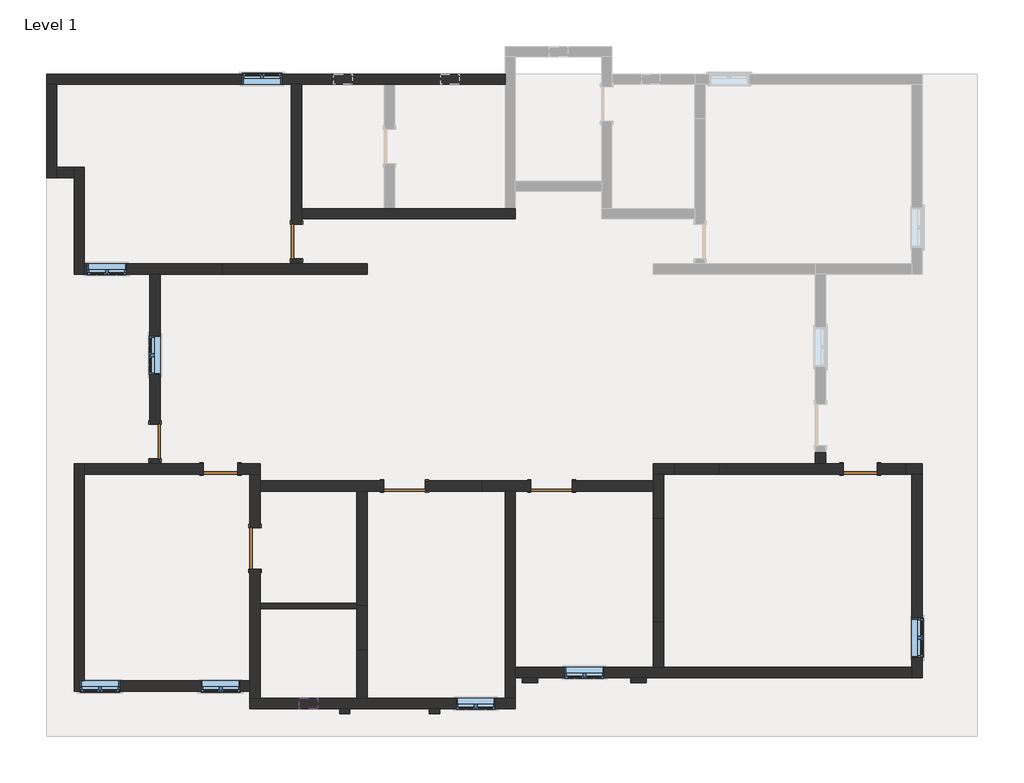
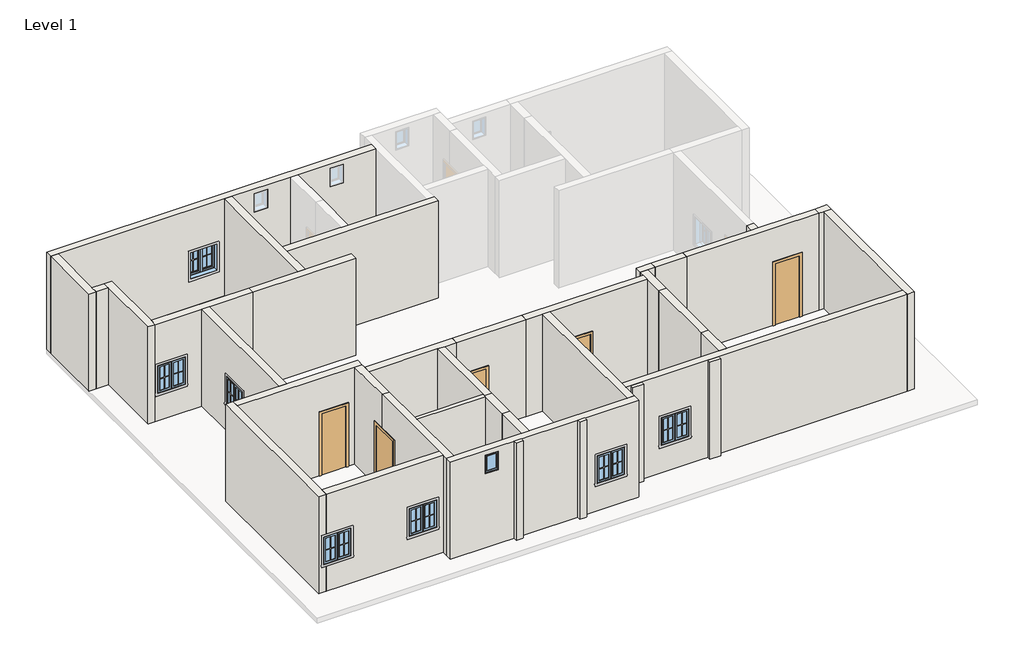
# One storey, part 1 of 2: 37 walls, 9 windows, 7 doors.
"""IFC4 building model written with IfcOpenShell, lengths in millimetres."""

from ifc_helpers import new_model, si_unit, frame, origin, origin_with_axes, place, context, project, spatial, polyline, outline, extrude, faceted_brep, transform, mapped, element, save
from components import door_a1484949, door_85036156, door_89fc3733, window_aa618e30, window_339605e1, window_791baf9d

model = new_model("IFC4")

# Units and contexts
model_context = context("Model", 3, world=origin())
ifc_project = project(units=[si_unit("LENGTHUNIT", "METRE", prefix="MILLI")], contexts=[model_context])

# Site, building, storey
site = spatial("IfcSite", under=ifc_project)
building = spatial("IfcBuilding", under=site)
storey = spatial("IfcBuildingStorey", under=building, Name="Level 1", Elevation=0.0)

# Doors
placement = place(None, origin())
door_shape = door_a1484949(model_context)
element("IfcDoor", 1, ObjectType="Single-Flush : 30\" x 80\"", at=placement, inside=storey, context=model_context, shape_type="MappedRepresentation", body=[
    mapped(door_shape, transform((-11694.6415084, -147.6064015, 0.0), x_axis=(0.0, -1.0, 0.0), y_axis=(1.0, 0.0, 0.0), z_axis=(0.0, 0.0, 1.0))),
])
door_2_shape = door_85036156(model_context)
element("IfcDoor", 2, ObjectType="Single-Flush : 30\" x 80\"", at=placement, inside=storey, context=model_context, shape_type="MappedRepresentation", body=[
    mapped(door_2_shape, transform((-8570.4415084, 4271.9935985, 0.0), x_axis=(0.0, -1.0, 0.0), y_axis=(1.0, 0.0, 0.0), z_axis=(0.0, 0.0, 1.0))),
])
element("IfcDoor", 3, ObjectType="Single-Flush : 30\" x 80\"", at=placement, inside=storey, context=model_context, shape_type="MappedRepresentation", body=[
    mapped(door_2_shape, transform((-10246.8415084, -757.2064015, 0.0), x_axis=(1.0, 0.0, 0.0), y_axis=(0.0, 1.0, 0.0), z_axis=(0.0, 0.0, 1.0))),
])
element("IfcDoor", 4, ObjectType="Single-Flush : 30\" x 80\"", at=placement, inside=storey, context=model_context, shape_type="MappedRepresentation", body=[
    mapped(door_2_shape, transform((3888.6257783, -757.2064015, 0.0), x_axis=(1.0, 0.0, 0.0), y_axis=(0.0, 1.0, 0.0), z_axis=(0.0, 0.0, 1.0))),
])
door_3_shape = door_89fc3733(model_context)
element("IfcDoor", 5, ObjectType="Single-Flush : 36\" x 80\"", at=placement, inside=storey, context=model_context, shape_type="MappedRepresentation", body=[
    mapped(door_3_shape, transform((-9484.8415084, -2515.5755761, 0.0), x_axis=(0.0, 1.0, 0.0), y_axis=(-1.0, 0.0, 0.0), z_axis=(0.0, 0.0, 1.0))),
])
element("IfcDoor", 6, ObjectType="Single-Flush : 36\" x 80\"", at=placement, inside=storey, context=model_context, shape_type="MappedRepresentation", body=[
    mapped(door_3_shape, transform((-6181.702216, -1138.2064015, 0.0), x_axis=(-1.0, 0.0, 0.0), y_axis=(0.0, -1.0, 0.0), z_axis=(0.0, 0.0, 1.0))),
])
element("IfcDoor", 7, ObjectType="Single-Flush : 36\" x 80\"", at=placement, inside=storey, context=model_context, shape_type="MappedRepresentation", body=[
    mapped(door_3_shape, transform((-2931.6415084, -1138.2064015, 0.0), x_axis=(-1.0, 0.0, 0.0), y_axis=(0.0, -1.0, 0.0), z_axis=(0.0, 0.0, 1.0))),
])

# Walls
element("IfcWall", 8, ObjectType="4.5\"", at=placement, inside=storey, context=model_context, shape_type="Brep", body=[
    faceted_brep([(-9370.5415084, -3843.3848078, 0.0), (-7236.9415084, -3843.3848078, 0.0), (-7236.9415084, -3843.3848078, 3200.4), (-9370.5415084, -3843.3848078, 3200.4), (-9370.5415084, -3729.0848078, 0.0), (-9370.5415084, -3729.0848078, 3200.4), (-7236.9415084, -3729.0848078, 3200.4), (-7236.9415084, -3729.0848078, 0.0), (-7236.9415084, -3786.2348078, 0.0), (-7236.9415084, -3786.2348078, 3200.4)], [[[0, 1, 2, 3]], [[4, 5, 6, 7]], [[1, 0, 4, 7, 8]], [[3, 2, 9, 6, 5]], [[2, 1, 8, 7, 6, 9]], [[0, 3, 5, 4]]]),
])
element("IfcWall", 9, ObjectType="4.5\"", at=placement, inside=storey, context=model_context, shape_type="SweptSolid", body=[
    extrude(outline(polyline([(-7389.3415084, -6167.4848078), (-7617.9415084, -6167.4848078), (-7617.9415084, -6053.1848078), (-7389.3415084, -6053.1848078), (-7389.3415084, -6167.4848078)])), origin_with_axes(), (0.0, 0.0, 1.0), 3200.4),
])
element("IfcWall", 10, ObjectType="4.5\"", at=placement, inside=storey, context=model_context, shape_type="SweptSolid", body=[
    extrude(outline(polyline([(-5408.1415084, -6167.4848078), (-5636.7415084, -6167.4848078), (-5636.7415084, -6053.1848078), (-5408.1415084, -6053.1848078), (-5408.1415084, -6167.4848078)])), origin_with_axes(), (0.0, 0.0, 1.0), 3200.4),
])
element("IfcWall", 11, ObjectType="4.5\"", at=placement, inside=storey, context=model_context, shape_type="SweptSolid", body=[
    extrude(outline(polyline([(-3236.4415084, -5481.6064015), (-3579.3415084, -5481.6064015), (-3579.3415084, -5367.3064015), (-3236.4415084, -5367.3064015), (-3236.4415084, -5481.6064015)])), origin_with_axes(), (0.0, 0.0, 1.0), 3200.4),
])
element("IfcWall", 12, ObjectType="4.5\"", at=placement, inside=storey, context=model_context, shape_type="SweptSolid", body=[
    extrude(outline(polyline([(-836.1415084, -5481.6064015), (-1179.0415084, -5481.6064015), (-1179.0415084, -5367.3064015), (-836.1415084, -5367.3064015), (-836.1415084, -5481.6064015)])), origin_with_axes(), (0.0, 0.0, 1.0), 3200.4),
])
element("IfcWall", 13, ObjectType="9\"", at=placement, inside=storey, context=model_context, shape_type="Brep", body=[
    faceted_brep([(-3960.3415084, 7967.6935985, 0.0), (-14094.9415084, 7967.6935985, 0.0), (-14094.9415084, 7967.6935985, 3200.4), (-3960.3415084, 7967.6935985, 3200.4), (-8900.6415084, 7967.6935985, 1828.8), (-9764.2415084, 7967.6935985, 1828.8), (-9764.2415084, 7967.6935985, 914.4), (-8900.6415084, 7967.6935985, 914.4), (-7338.5415084, 7967.6935985, 3048.0), (-7744.9415084, 7967.6935985, 3048.0), (-7744.9415084, 7967.6935985, 2438.4), (-7338.5415084, 7967.6935985, 2438.4), (-4976.3415084, 7967.6935985, 3048.0), (-5382.7415084, 7967.6935985, 3048.0), (-5382.7415084, 7967.6935985, 2438.4), (-4976.3415084, 7967.6935985, 2438.4), (-3960.3415084, 7739.0935985, 0.0), (-3960.3415084, 7739.0935985, 3200.4), (-6398.7415084, 7739.0935985, 3200.4), (-6627.3415084, 7739.0935985, 3200.4), (-8456.1415084, 7739.0935985, 3200.4), (-8684.7415084, 7739.0935985, 3200.4), (-13866.3415084, 7739.0935985, 3200.4), (-14094.9415084, 7739.0935985, 3200.4), (-14094.9415084, 7739.0935985, 0.0), (-13866.3415084, 7739.0935985, 0.0), (-8684.7415084, 7739.0935985, 0.0), (-8456.1415084, 7739.0935985, 0.0), (-6627.3415084, 7739.0935985, 0.0), (-6398.7415084, 7739.0935985, 0.0), (-8900.6415084, 7739.0935985, 1828.8), (-8900.6415084, 7739.0935985, 914.4), (-9764.2415084, 7739.0935985, 914.4), (-9764.2415084, 7739.0935985, 1828.8), (-7338.5415084, 7739.0935985, 3048.0), (-7338.5415084, 7739.0935985, 2438.4), (-7744.9415084, 7739.0935985, 2438.4), (-7744.9415084, 7739.0935985, 3048.0), (-4976.3415084, 7739.0935985, 3048.0), (-4976.3415084, 7739.0935985, 2438.4), (-5382.7415084, 7739.0935985, 2438.4), (-5382.7415084, 7739.0935985, 3048.0)], [[[0, 1, 2, 3], [4, 5, 6, 7], [8, 9, 10, 11], [12, 13, 14, 15]], [[16, 17, 18, 19, 20, 21, 22, 23, 24, 25, 26, 27, 28, 29], [30, 31, 32, 33], [34, 35, 36, 37], [38, 39, 40, 41]], [[1, 0, 16, 29, 28, 27, 26, 25, 24]], [[3, 2, 23, 22, 21, 20, 19, 18, 17]], [[2, 1, 24, 23]], [[0, 3, 17, 16]], [[31, 30, 4, 7]], [[32, 31, 7, 6]], [[33, 32, 6, 5]], [[30, 33, 5, 4]], [[35, 34, 8, 11]], [[36, 35, 11, 10]], [[37, 36, 10, 9]], [[34, 37, 9, 8]], [[39, 38, 12, 15]], [[40, 39, 15, 14]], [[41, 40, 14, 13]], [[38, 41, 13, 12]]]),
])
element("IfcWall", 14, ObjectType="9\"", at=placement, inside=storey, context=model_context, shape_type="Brep", body=[
    faceted_brep([(-14094.9415084, 7739.0935985, 0.0), (-14094.9415084, 5681.6935985, 0.0), (-14094.9415084, 5681.6935985, 3200.4), (-14094.9415084, 7739.0935985, 3200.4), (-13866.3415084, 7739.0935985, 0.0), (-13866.3415084, 7739.0935985, 3200.4), (-13866.3415084, 5910.2935985, 3200.4), (-13866.3415084, 5681.6935985, 3200.4), (-13866.3415084, 5681.6935985, 0.0), (-13866.3415084, 5910.2935985, 0.0)], [[[0, 1, 2, 3]], [[4, 5, 6, 7, 8, 9]], [[1, 0, 4, 9, 8]], [[3, 2, 7, 6, 5]], [[0, 3, 5, 4]], [[2, 1, 8, 7]]]),
])
element("IfcWall", 15, ObjectType="9\"", at=placement, inside=storey, context=model_context, shape_type="Brep", body=[
    faceted_brep([(-13485.3415084, 5910.2935985, 0.0), (-13485.3415084, 5681.6935985, 0.0), (-13485.3415084, 3548.0935985, 0.0), (-13485.3415084, 3548.0935985, 3200.4), (-13485.3415084, 5681.6935985, 3200.4), (-13485.3415084, 5910.2935985, 3200.4), (-13256.7415084, 5910.2935985, 0.0), (-13256.7415084, 5910.2935985, 3200.4), (-13256.7415084, 3776.6935985, 3200.4), (-13256.7415084, 3548.0935985, 3200.4), (-13256.7415084, 3548.0935985, 0.0), (-13256.7415084, 3776.6935985, 0.0)], [[[0, 1, 2, 3, 4, 5]], [[6, 7, 8, 9, 10, 11]], [[2, 1, 0, 6, 11, 10]], [[5, 4, 3, 9, 8, 7]], [[0, 5, 7, 6]], [[3, 2, 10, 9]]]),
])
element("IfcWall", 16, ObjectType="9\"", at=placement, inside=storey, context=model_context, shape_type="SweptSolid", body=[
    extrude(outline(polyline([(-13866.3415084, 5910.2935985), (-13485.3415084, 5910.2935985), (-13485.3415084, 5681.6935985), (-13866.3415084, 5681.6935985), (-13866.3415084, 5910.2935985)])), origin_with_axes(), (0.0, 0.0, 1.0), 3200.4),
])
element("IfcWall", 17, ObjectType="9\"", at=placement, inside=storey, context=model_context, shape_type="Brep", body=[
    faceted_brep([(-7008.3415084, 3776.6935985, 0.0), (-8456.1415084, 3776.6935985, 0.0), (-8684.7415084, 3776.6935985, 0.0), (-10214.9670183, 3776.6935985, 0.0), (-10214.9670183, 3776.6935985, 3200.4), (-8684.7415084, 3776.6935985, 3200.4), (-8456.1415084, 3776.6935985, 3200.4), (-7008.3415084, 3776.6935985, 3200.4), (-7008.3415084, 3548.0935985, 0.0), (-7008.3415084, 3548.0935985, 3200.4), (-10214.9670183, 3548.0935985, 3200.4), (-10214.9670183, 3548.0935985, 0.0)], [[[0, 1, 2, 3, 4, 5, 6, 7]], [[8, 9, 10, 11]], [[3, 2, 1, 0, 8, 11]], [[4, 3, 11, 10]], [[7, 6, 5, 4, 10, 9]], [[0, 7, 9, 8]]]),
])
element("IfcWall", 18, ObjectType="9\"", at=placement, inside=storey, context=model_context, shape_type="Brep", body=[
    faceted_brep([(-10214.9670183, 3776.6935985, 0.0), (-13256.7415084, 3776.6935985, 0.0), (-13256.7415084, 3776.6935985, 3200.4), (-10214.9670183, 3776.6935985, 3200.4), (-13193.2415084, 3776.6935985, 1828.8), (-13193.2415084, 3776.6935985, 914.4), (-12329.6415084, 3776.6935985, 914.4), (-12329.6415084, 3776.6935985, 1828.8), (-10214.9670183, 3548.0935985, 0.0), (-10214.9670183, 3548.0935985, 3200.4), (-11580.3415084, 3548.0935985, 3200.4), (-11808.9415084, 3548.0935985, 3200.4), (-13256.7415084, 3548.0935985, 3200.4), (-13256.7415084, 3548.0935985, 0.0), (-11808.9415084, 3548.0935985, 0.0), (-11580.3415084, 3548.0935985, 0.0), (-13193.2415084, 3548.0935985, 1828.8), (-12329.6415084, 3548.0935985, 1828.8), (-12329.6415084, 3548.0935985, 914.4), (-13193.2415084, 3548.0935985, 914.4)], [[[0, 1, 2, 3], [4, 5, 6, 7]], [[8, 9, 10, 11, 12, 13, 14, 15], [16, 17, 18, 19]], [[1, 0, 8, 15, 14, 13]], [[3, 2, 12, 11, 10, 9]], [[0, 3, 9, 8]], [[2, 1, 13, 12]], [[5, 4, 16, 19]], [[6, 5, 19, 18]], [[7, 6, 18, 17]], [[4, 7, 17, 16]]]),
])
element("IfcWall", 19, ObjectType="9\"", at=placement, inside=storey, context=model_context, shape_type="SweptSolid", body=[
    extrude(outline(polyline([(-528.6064015, 2032.0), (-528.6064015, 0.0), (-642.9064015, 0.0), (-642.9064015, 3200.4), (3548.0935985, 3200.4), (3548.0935985, 0.0), (233.3935985, 0.0), (233.3935985, 2032.0), (-528.6064015, 2032.0)]), holes=[polyline([(2189.1935985, 1828.8), (1325.5935985, 1828.8), (1325.5935985, 914.4), (2189.1935985, 914.4), (2189.1935985, 1828.8)])]), frame((-11808.9415084, 0.0, 0.0), z_axis=(1.0, 0.0, 0.0), x_axis=(0.0, 1.0, 0.0)), (0.0, 0.0, 1.0), 228.6),
])
element("IfcWall", 20, ObjectType="9\"", at=placement, inside=storey, context=model_context, shape_type="Brep", body=[
    faceted_brep([(-13485.3415084, -642.9064015, 0.0), (-13485.3415084, -5672.1064015, 0.0), (-13485.3415084, -5672.1064015, 3200.4), (-13485.3415084, -642.9064015, 3200.4), (-13256.7415084, -5672.1064015, 0.0), (-13256.7415084, -5443.5064015, 0.0), (-13256.7415084, -871.5064015, 0.0), (-13256.7415084, -642.9064015, 0.0), (-13256.7415084, -642.9064015, 3200.4), (-13256.7415084, -871.5064015, 3200.4), (-13256.7415084, -5443.5064015, 3200.4), (-13256.7415084, -5672.1064015, 3200.4), (-13256.7415084, -5672.1064015, 1828.8), (-13256.7415084, -5443.5064015, 1828.8), (-13256.7415084, -5443.5064015, 914.4), (-13256.7415084, -5672.1064015, 914.4), (-13345.6415084, -5672.1064015, 914.4), (-13345.6415084, -5672.1064015, 1828.8), (-13345.6415084, -5443.5064015, 1828.8), (-13345.6415084, -5443.5064015, 914.4)], [[[0, 1, 2, 3]], [[4, 5, 6, 7, 8, 9, 10, 11, 12, 13, 14, 15]], [[1, 0, 7, 6, 5, 4]], [[3, 2, 11, 10, 9, 8]], [[2, 1, 4, 15, 16, 17, 12, 11]], [[0, 3, 8, 7]], [[18, 19, 14, 13]], [[19, 18, 17, 16]], [[19, 16, 15, 14]], [[17, 18, 13, 12]]]),
])
element("IfcWall", 21, ObjectType="9\"", at=placement, inside=storey, context=model_context, shape_type="Brep", body=[
    faceted_brep([(-3731.7415084, 4995.8935985, 0.0), (-3960.3415084, 4995.8935985, 0.0), (-6398.7415084, 4995.8935985, 0.0), (-6627.3415084, 4995.8935985, 0.0), (-8456.1415084, 4995.8935985, 0.0), (-8456.1415084, 4995.8935985, 3200.4), (-6627.3415084, 4995.8935985, 3200.4), (-6398.7415084, 4995.8935985, 3200.4), (-3960.3415084, 4995.8935985, 3200.4), (-3731.7415084, 4995.8935985, 3200.4), (-3731.7415084, 4767.2935985, 0.0), (-3731.7415084, 4767.2935985, 3200.4), (-8456.1415084, 4767.2935985, 3200.4), (-8456.1415084, 4767.2935985, 0.0)], [[[0, 1, 2, 3, 4, 5, 6, 7, 8, 9]], [[10, 11, 12, 13]], [[4, 3, 2, 1, 0, 10, 13]], [[9, 8, 7, 6, 5, 12, 11]], [[0, 9, 11, 10]], [[5, 4, 13, 12]]]),
])
element("IfcWall", 22, ObjectType="9\"", at=placement, inside=storey, context=model_context, shape_type="Brep", body=[
    faceted_brep([(-8684.7415084, 3890.9935985, 2032.0), (-8684.7415084, 3890.9935985, 0.0), (-8684.7415084, 3776.6935985, 0.0), (-8684.7415084, 3776.6935985, 3200.4), (-8684.7415084, 7739.0935985, 3200.4), (-8684.7415084, 7739.0935985, 0.0), (-8684.7415084, 4652.9935985, 0.0), (-8684.7415084, 4652.9935985, 2032.0), (-8456.1415084, 3776.6935985, 0.0), (-8456.1415084, 3890.9935985, 0.0), (-8456.1415084, 3890.9935985, 2032.0), (-8456.1415084, 4652.9935985, 2032.0), (-8456.1415084, 4652.9935985, 0.0), (-8456.1415084, 4767.2935985, 0.0), (-8456.1415084, 4995.8935985, 0.0), (-8456.1415084, 7739.0935985, 0.0), (-8456.1415084, 7739.0935985, 3200.4), (-8456.1415084, 4995.8935985, 3200.4), (-8456.1415084, 4767.2935985, 3200.4), (-8456.1415084, 3776.6935985, 3200.4)], [[[0, 1, 2, 3, 4, 5, 6, 7]], [[8, 9, 10, 11, 12, 13, 14, 15, 16, 17, 18, 19]], [[6, 5, 15, 14, 13, 12]], [[2, 1, 9, 8]], [[4, 3, 19, 18, 17, 16]], [[5, 4, 16, 15]], [[3, 2, 8, 19]], [[10, 9, 1, 0]], [[11, 10, 0, 7]], [[12, 11, 7, 6]]]),
])
element("IfcWall", 23, ObjectType="9\"", at=placement, inside=storey, context=model_context, shape_type="Brep", body=[
    faceted_brep([(-6638.902216, -1023.9064015, 0.0), (-9370.5415084, -1023.9064015, 0.0), (-9370.5415084, -1023.9064015, 3200.4), (-6638.902216, -1023.9064015, 3200.4), (-6638.902216, -1023.9064015, 2032.0), (-6638.902216, -1252.5064015, 0.0), (-6638.902216, -1252.5064015, 2032.0), (-6638.902216, -1252.5064015, 3200.4), (-7008.3415084, -1252.5064015, 3200.4), (-7236.9415084, -1252.5064015, 3200.4), (-9370.5415084, -1252.5064015, 3200.4), (-9370.5415084, -1252.5064015, 0.0), (-7236.9415084, -1252.5064015, 0.0), (-7008.3415084, -1252.5064015, 0.0)], [[[0, 1, 2, 3, 4]], [[5, 6, 7, 8, 9, 10, 11, 12, 13]], [[1, 0, 5, 13, 12, 11]], [[3, 2, 10, 9, 8, 7]], [[0, 4, 3, 7, 6, 5]], [[2, 1, 11, 10]]]),
])
element("IfcWall", 24, ObjectType="9\"", at=placement, inside=storey, context=model_context, shape_type="SweptSolid", body=[
    extrude(outline(polyline([(0.0, -13256.7415084), (0.0, -9599.1415084), (3200.4, -9599.1415084), (3200.4, -13256.7415084), (1828.8, -13256.7415084), (1828.8, -12482.0415084), (914.4, -12482.0415084), (914.4, -13256.7415084), (0.0, -13256.7415084)]), holes=[polyline([(1828.8, -10678.6415084), (1828.8, -9815.0415084), (914.4, -9815.0415084), (914.4, -10678.6415084), (1828.8, -10678.6415084)])]), frame((0.0, -5672.1064015, 0.0), z_axis=(0.0, 1.0, 0.0), x_axis=(0.0, 0.0, 1.0)), (0.0, 0.0, 1.0), 228.6),
])
element("IfcWall", 25, ObjectType="9\"", at=placement, inside=storey, context=model_context, shape_type="Brep", body=[
    faceted_brep([(-3731.7415084, -5824.5848078, 0.0), (-3960.3415084, -5824.5848078, 0.0), (-7008.3415084, -5824.5848078, 0.0), (-7236.9415084, -5824.5848078, 0.0), (-9370.5415084, -5824.5848078, 0.0), (-9599.1415084, -5824.5848078, 0.0), (-9599.1415084, -5824.5848078, 3200.4), (-9370.5415084, -5824.5848078, 3200.4), (-7236.9415084, -5824.5848078, 3200.4), (-7008.3415084, -5824.5848078, 3200.4), (-3960.3415084, -5824.5848078, 3200.4), (-3731.7415084, -5824.5848078, 3200.4), (-5039.8415084, -5824.5848078, 1828.8), (-5039.8415084, -5824.5848078, 914.4), (-4176.2415084, -5824.5848078, 914.4), (-4176.2415084, -5824.5848078, 1828.8), (-8506.9415084, -5824.5848078, 3048.0), (-8506.9415084, -5824.5848078, 2438.4), (-8100.5415084, -5824.5848078, 2438.4), (-8100.5415084, -5824.5848078, 3048.0), (-3731.7415084, -6053.1848078, 0.0), (-3731.7415084, -6053.1848078, 3200.4), (-9599.1415084, -6053.1848078, 3200.4), (-9599.1415084, -6053.1848078, 0.0), (-5039.8415084, -6053.1848078, 1828.8), (-4176.2415084, -6053.1848078, 1828.8), (-4176.2415084, -6053.1848078, 914.4), (-5039.8415084, -6053.1848078, 914.4), (-8506.9415084, -6053.1848078, 3048.0), (-8100.5415084, -6053.1848078, 3048.0), (-8100.5415084, -6053.1848078, 2438.4), (-8506.9415084, -6053.1848078, 2438.4)], [[[0, 1, 2, 3, 4, 5, 6, 7, 8, 9, 10, 11], [12, 13, 14, 15], [16, 17, 18, 19]], [[20, 21, 22, 23], [24, 25, 26, 27], [28, 29, 30, 31]], [[5, 4, 3, 2, 1, 0, 20, 23]], [[11, 10, 9, 8, 7, 6, 22, 21]], [[6, 5, 23, 22]], [[0, 11, 21, 20]], [[13, 12, 24, 27]], [[14, 13, 27, 26]], [[15, 14, 26, 25]], [[12, 15, 25, 24]], [[17, 16, 28, 31]], [[18, 17, 31, 30]], [[19, 18, 30, 29]], [[16, 19, 29, 28]]]),
])
element("IfcWall", 26, ObjectType="9\"", at=placement, inside=storey, context=model_context, shape_type="SweptSolid", body=[
    extrude(outline(polyline([(-7236.9415084, -5824.5848078), (-7236.9415084, -4769.1468823), (-7008.3415084, -4769.1468823), (-7008.3415084, -5824.5848078), (-7236.9415084, -5824.5848078)])), origin_with_axes(), (0.0, 0.0, 1.0), 3200.4),
])
element("IfcWall", 27, ObjectType="9\"", at=placement, inside=storey, context=model_context, shape_type="Brep", body=[
    faceted_brep([(-7236.9415084, -3786.2348078, 0.0), (-7236.9415084, -3843.3848078, 0.0), (-7236.9415084, -4769.1468823, 0.0), (-7236.9415084, -4769.1468823, 3200.4), (-7236.9415084, -3843.3848078, 3200.4), (-7236.9415084, -3786.2348078, 3200.4), (-7008.3415084, -3786.2348078, 0.0), (-7008.3415084, -3786.2348078, 3200.4), (-7008.3415084, -4769.1468823, 3200.4), (-7008.3415084, -4769.1468823, 0.0)], [[[0, 1, 2, 3, 4, 5]], [[6, 7, 8, 9]], [[2, 1, 0, 6, 9]], [[3, 2, 9, 8]], [[5, 4, 3, 8, 7]], [[0, 5, 7, 6]]]),
])
element("IfcWall", 28, ObjectType="9\"", at=placement, inside=storey, context=model_context, shape_type="Brep", body=[
    faceted_brep([(-7236.9415084, -1252.5064015, 0.0), (-7236.9415084, -3729.0848078, 0.0), (-7236.9415084, -3786.2348078, 0.0), (-7236.9415084, -3786.2348078, 3200.4), (-7236.9415084, -3729.0848078, 3200.4), (-7236.9415084, -1252.5064015, 3200.4), (-7008.3415084, -1252.5064015, 0.0), (-7008.3415084, -1252.5064015, 3200.4), (-7008.3415084, -3786.2348078, 3200.4), (-7008.3415084, -3786.2348078, 0.0)], [[[0, 1, 2, 3, 4, 5]], [[6, 7, 8, 9]], [[2, 1, 0, 6, 9]], [[3, 2, 9, 8]], [[5, 4, 3, 8, 7]], [[0, 5, 7, 6]]]),
])
element("IfcWall", 29, ObjectType="9\"", at=placement, inside=storey, context=model_context, shape_type="SweptSolid", body=[
    extrude(outline(polyline([(3200.4, -4471.5671604), (3200.4, -6638.902216), (2032.0, -6638.902216), (2032.0, -5724.502216), (0.0, -5724.502216), (0.0, -4471.5671604), (3200.4, -4471.5671604)])), frame((0.0, -1252.5064015, 0.0), z_axis=(0.0, 1.0, 0.0), x_axis=(0.0, 0.0, 1.0)), (0.0, 0.0, 1.0), 228.6),
])
element("IfcWall", 30, ObjectType="9\"", at=placement, inside=storey, context=model_context, shape_type="Brep", body=[
    faceted_brep([(-3388.8415084, -1023.9064015, 2032.0), (-3388.8415084, -1023.9064015, 0.0), (-4471.5671604, -1023.9064015, 0.0), (-4471.5671604, -1023.9064015, 3200.4), (-683.7415084, -1023.9064015, 3200.4), (-683.7415084, -1023.9064015, 0.0), (-2474.4415084, -1023.9064015, 0.0), (-2474.4415084, -1023.9064015, 2032.0), (-4471.5671604, -1252.5064015, 0.0), (-3960.3415084, -1252.5064015, 0.0), (-3731.7415084, -1252.5064015, 0.0), (-3388.8415084, -1252.5064015, 0.0), (-3388.8415084, -1252.5064015, 2032.0), (-2474.4415084, -1252.5064015, 2032.0), (-2474.4415084, -1252.5064015, 0.0), (-683.7415084, -1252.5064015, 0.0), (-683.7415084, -1252.5064015, 3200.4), (-3731.7415084, -1252.5064015, 3200.4), (-3960.3415084, -1252.5064015, 3200.4), (-4471.5671604, -1252.5064015, 3200.4)], [[[0, 1, 2, 3, 4, 5, 6, 7]], [[8, 9, 10, 11, 12, 13, 14, 15, 16, 17, 18, 19]], [[6, 5, 15, 14]], [[2, 1, 11, 10, 9, 8]], [[3, 2, 8, 19]], [[4, 3, 19, 18, 17, 16]], [[5, 4, 16, 15]], [[12, 11, 1, 0]], [[13, 12, 0, 7]], [[14, 13, 7, 6]]]),
])
element("IfcWall", 31, ObjectType="9\"", at=placement, inside=storey, context=model_context, shape_type="Brep", body=[
    faceted_brep([(5031.2584916, -871.5064015, 0.0), (5031.2584916, -5138.7064015, 0.0), (5031.2584916, -5367.3064015, 0.0), (5031.2584916, -5367.3064015, 3200.4), (5031.2584916, -5138.7064015, 3200.4), (5031.2584916, -871.5064015, 3200.4), (5031.2584916, -4922.8064015, 1828.8), (5031.2584916, -4922.8064015, 914.4), (5031.2584916, -4059.2064015, 914.4), (5031.2584916, -4059.2064015, 1828.8), (5259.8584916, -871.5064015, 0.0), (5259.8584916, -871.5064015, 3200.4), (5259.8584916, -5367.3064015, 3200.4), (5259.8584916, -5367.3064015, 0.0), (5259.8584916, -4922.8064015, 1828.8), (5259.8584916, -4059.2064015, 1828.8), (5259.8584916, -4059.2064015, 914.4), (5259.8584916, -4922.8064015, 914.4)], [[[0, 1, 2, 3, 4, 5], [6, 7, 8, 9]], [[10, 11, 12, 13], [14, 15, 16, 17]], [[2, 1, 0, 10, 13]], [[5, 4, 3, 12, 11]], [[3, 2, 13, 12]], [[0, 5, 11, 10]], [[7, 6, 14, 17]], [[8, 7, 17, 16]], [[9, 8, 16, 15]], [[6, 9, 15, 14]]]),
])
element("IfcWall", 32, ObjectType="9\"", at=placement, inside=storey, context=model_context, shape_type="Brep", body=[
    faceted_brep([(5031.2584916, -5138.7064015, 0.0), (-455.1415084, -5138.7064015, 0.0), (-683.7415084, -5138.7064015, 0.0), (-3731.7415084, -5138.7064015, 0.0), (-3731.7415084, -5138.7064015, 3200.4), (-683.7415084, -5138.7064015, 3200.4), (-455.1415084, -5138.7064015, 3200.4), (5031.2584916, -5138.7064015, 3200.4), (-1775.9415084, -5138.7064015, 1828.8), (-2639.5415084, -5138.7064015, 1828.8), (-2639.5415084, -5138.7064015, 914.4), (-1775.9415084, -5138.7064015, 914.4), (5031.2584916, -5367.3064015, 0.0), (5031.2584916, -5367.3064015, 3200.4), (-3731.7415084, -5367.3064015, 3200.4), (-3731.7415084, -5367.3064015, 0.0), (-1775.9415084, -5367.3064015, 1828.8), (-1775.9415084, -5367.3064015, 914.4), (-2639.5415084, -5367.3064015, 914.4), (-2639.5415084, -5367.3064015, 1828.8)], [[[0, 1, 2, 3, 4, 5, 6, 7], [8, 9, 10, 11]], [[12, 13, 14, 15], [16, 17, 18, 19]], [[3, 2, 1, 0, 12, 15]], [[7, 6, 5, 4, 14, 13]], [[0, 7, 13, 12]], [[4, 3, 15, 14]], [[17, 16, 8, 11]], [[18, 17, 11, 10]], [[19, 18, 10, 9]], [[16, 19, 9, 8]]]),
])
element("IfcWall", 33, ObjectType="9\"", at=placement, inside=storey, context=model_context, shape_type="Brep", body=[
    faceted_brep([(-9370.5415084, -642.9064015, 0.0), (-9865.8415084, -642.9064015, 0.0), (-9865.8415084, -642.9064015, 2032.0), (-10627.8415084, -642.9064015, 2032.0), (-10627.8415084, -642.9064015, 0.0), (-11580.3415084, -642.9064015, 0.0), (-11808.9415084, -642.9064015, 0.0), (-13256.7415084, -642.9064015, 0.0), (-13256.7415084, -642.9064015, 3200.4), (-11808.9415084, -642.9064015, 3200.4), (-11580.3415084, -642.9064015, 3200.4), (-9370.5415084, -642.9064015, 3200.4), (-9865.8415084, -871.5064015, 2032.0), (-9865.8415084, -871.5064015, 0.0), (-9599.1415084, -871.5064015, 0.0), (-9370.5415084, -871.5064015, 0.0), (-9370.5415084, -871.5064015, 3200.4), (-9599.1415084, -871.5064015, 3200.4), (-13256.7415084, -871.5064015, 3200.4), (-13256.7415084, -871.5064015, 0.0), (-10627.8415084, -871.5064015, 0.0), (-10627.8415084, -871.5064015, 2032.0)], [[[0, 1, 2, 3, 4, 5, 6, 7, 8, 9, 10, 11]], [[12, 13, 14, 15, 16, 17, 18, 19, 20, 21]], [[20, 19, 7, 6, 5, 4]], [[15, 14, 13, 1, 0]], [[11, 10, 9, 8, 18, 17, 16]], [[8, 7, 19, 18]], [[0, 11, 16, 15]], [[2, 1, 13, 12]], [[3, 2, 12, 21]], [[4, 3, 21, 20]]]),
])
element("IfcWall", 34, ObjectType="9\"", at=placement, inside=storey, context=model_context, shape_type="Brep", body=[
    faceted_brep([(-9370.5415084, -871.5064015, 3200.4), (-9370.5415084, -1023.9064015, 3200.4), (-9370.5415084, -1252.5064015, 3200.4), (-9370.5415084, -2363.1755761, 3200.4), (-9370.5415084, -2363.1755761, 2032.0), (-9370.5415084, -2058.3755761, 2032.0), (-9370.5415084, -2058.3755761, 0.0), (-9370.5415084, -1252.5064015, 0.0), (-9370.5415084, -1023.9064015, 0.0), (-9370.5415084, -871.5064015, 0.0), (-9599.1415084, -2363.1755761, 3200.4), (-9599.1415084, -871.5064015, 3200.4), (-9599.1415084, -871.5064015, 0.0), (-9599.1415084, -2058.3755761, 0.0), (-9599.1415084, -2058.3755761, 2032.0), (-9599.1415084, -2363.1755761, 2032.0)], [[[0, 1, 2, 3, 4, 5, 6, 7, 8, 9]], [[10, 11, 12, 13, 14, 15]], [[12, 9, 8, 7, 6, 13]], [[3, 2, 1, 0, 11, 10]], [[3, 10, 15, 4]], [[0, 9, 12, 11]], [[5, 14, 13, 6]], [[14, 5, 4, 15]]]),
])
element("IfcWall", 35, ObjectType="9\"", at=placement, inside=storey, context=model_context, shape_type="Brep", body=[
    faceted_brep([(-9599.1415084, -5824.5848078, 3200.4), (-9599.1415084, -5672.1064015, 3200.4), (-9599.1415084, -5443.5064015, 3200.4), (-9599.1415084, -2363.1755761, 3200.4), (-9599.1415084, -2363.1755761, 2032.0), (-9599.1415084, -2972.7755761, 2032.0), (-9599.1415084, -2972.7755761, 0.0), (-9599.1415084, -5443.5064015, 0.0), (-9599.1415084, -5672.1064015, 0.0), (-9599.1415084, -5824.5848078, 0.0), (-9370.5415084, -2363.1755761, 3200.4), (-9370.5415084, -3729.0848078, 3200.4), (-9370.5415084, -3843.3848078, 3200.4), (-9370.5415084, -5824.5848078, 3200.4), (-9370.5415084, -5824.5848078, 0.0), (-9370.5415084, -3843.3848078, 0.0), (-9370.5415084, -3729.0848078, 0.0), (-9370.5415084, -2972.7755761, 0.0), (-9370.5415084, -2972.7755761, 2032.0), (-9370.5415084, -2363.1755761, 2032.0)], [[[0, 1, 2, 3, 4, 5, 6, 7, 8, 9]], [[10, 11, 12, 13, 14, 15, 16, 17, 18, 19]], [[14, 9, 8, 7, 6, 17, 16, 15]], [[3, 2, 1, 0, 13, 12, 11, 10]], [[3, 10, 19, 4]], [[0, 9, 14, 13]], [[18, 5, 4, 19]], [[5, 18, 17, 6]]]),
])
element("IfcWall", 36, ObjectType="9\"", at=placement, inside=storey, context=model_context, shape_type="Brep", body=[
    faceted_brep([(-3731.7415084, -5824.5848078, 0.0), (-3731.7415084, -5367.3064015, 0.0), (-3731.7415084, -5138.7064015, 0.0), (-3731.7415084, -1252.5064015, 0.0), (-3731.7415084, -1252.5064015, 3200.4), (-3731.7415084, -5138.7064015, 3200.4), (-3731.7415084, -5367.3064015, 3200.4), (-3731.7415084, -5824.5848078, 3200.4), (-3960.3415084, -5824.5848078, 0.0), (-3960.3415084, -5824.5848078, 3200.4), (-3960.3415084, -1252.5064015, 3200.4), (-3960.3415084, -1252.5064015, 0.0)], [[[0, 1, 2, 3, 4, 5, 6, 7]], [[8, 9, 10, 11]], [[3, 2, 1, 0, 8, 11]], [[7, 6, 5, 4, 10, 9]], [[0, 7, 9, 8]], [[4, 3, 11, 10]]]),
])
element("IfcWall", 37, ObjectType="9\"", at=placement, inside=storey, context=model_context, shape_type="SweptSolid", body=[
    extrude(outline(polyline([(2897.6584916, -642.9064015), (2897.6584916, -396.999146), (3126.2584916, -396.999146), (3126.2584916, -642.9064015), (2897.6584916, -642.9064015)])), origin_with_axes(), (0.0, 0.0, 1.0), 3200.4),
])
element("IfcWall", 38, ObjectType="9\"", at=placement, inside=storey, context=model_context, shape_type="Brep", body=[
    faceted_brep([(5259.8584916, -642.9064015, 0.0), (4879.593065, -642.9064015, 0.0), (4879.593065, -642.9064015, 3200.4), (5259.8584916, -642.9064015, 3200.4), (5259.8584916, -871.5064015, 0.0), (5259.8584916, -871.5064015, 3200.4), (5031.2584916, -871.5064015, 3200.4), (4879.593065, -871.5064015, 3200.4), (4879.593065, -871.5064015, 0.0), (5031.2584916, -871.5064015, 0.0)], [[[0, 1, 2, 3]], [[4, 5, 6, 7, 8, 9]], [[1, 0, 4, 9, 8]], [[2, 1, 8, 7]], [[3, 2, 7, 6, 5]], [[0, 3, 5, 4]]]),
])
element("IfcWall", 39, ObjectType="9\"", at=placement, inside=storey, context=model_context, shape_type="SweptSolid", body=[
    extrude(outline(polyline([(-226.5415084, -642.9064015), (764.0584916, -642.9064015), (764.0584916, -871.5064015), (-226.5415084, -871.5064015), (-226.5415084, -642.9064015)])), origin_with_axes(), (0.0, 0.0, 1.0), 3200.4),
])
element("IfcWall", 40, ObjectType="9\"", at=placement, inside=storey, context=model_context, shape_type="Brep", body=[
    faceted_brep([(-226.5415084, -642.9064015, 0.0), (-683.7415084, -642.9064015, 0.0), (-683.7415084, -642.9064015, 3200.4), (-226.5415084, -642.9064015, 3200.4), (-226.5415084, -871.5064015, 0.0), (-226.5415084, -871.5064015, 3200.4), (-455.1415084, -871.5064015, 3200.4), (-683.7415084, -871.5064015, 3200.4), (-683.7415084, -871.5064015, 0.0), (-455.1415084, -871.5064015, 0.0)], [[[0, 1, 2, 3]], [[4, 5, 6, 7, 8, 9]], [[1, 0, 4, 9, 8]], [[3, 2, 7, 6, 5]], [[0, 3, 5, 4]], [[2, 1, 8, 7]]]),
])
element("IfcWall", 41, ObjectType="9\"", at=placement, inside=storey, context=model_context, shape_type="SweptSolid", body=[
    extrude(outline(polyline([(-683.7415084, -5138.7064015), (-683.7415084, -4148.1064015), (-455.1415084, -4148.1064015), (-455.1415084, -5138.7064015), (-683.7415084, -5138.7064015)])), origin_with_axes(), (0.0, 0.0, 1.0), 3200.4),
])
element("IfcWall", 42, ObjectType="9\"", at=placement, inside=storey, context=model_context, shape_type="SweptSolid", body=[
    extrude(outline(polyline([(-683.7415084, -4148.1064015), (-683.7415084, -1862.1064015), (-455.1415084, -1862.1064015), (-455.1415084, -4148.1064015), (-683.7415084, -4148.1064015)])), origin_with_axes(), (0.0, 0.0, 1.0), 3200.4),
])
element("IfcWall", 43, ObjectType="9\"", at=placement, inside=storey, context=model_context, shape_type="Brep", body=[
    faceted_brep([(-683.7415084, -871.5064015, 0.0), (-683.7415084, -1023.9064015, 0.0), (-683.7415084, -1252.5064015, 0.0), (-683.7415084, -1862.1064015, 0.0), (-683.7415084, -1862.1064015, 3200.4), (-683.7415084, -1252.5064015, 3200.4), (-683.7415084, -1023.9064015, 3200.4), (-683.7415084, -871.5064015, 3200.4), (-455.1415084, -871.5064015, 0.0), (-455.1415084, -871.5064015, 3200.4), (-455.1415084, -1862.1064015, 3200.4), (-455.1415084, -1862.1064015, 0.0)], [[[0, 1, 2, 3, 4, 5, 6, 7]], [[8, 9, 10, 11]], [[3, 2, 1, 0, 8, 11]], [[4, 3, 11, 10]], [[7, 6, 5, 4, 10, 9]], [[0, 7, 9, 8]]]),
])
element("IfcWall", 44, ObjectType="9\"", at=placement, inside=storey, context=model_context, shape_type="Brep", body=[
    faceted_brep([(4879.593065, -642.9064015, 0.0), (4269.6257783, -642.9064015, 0.0), (4269.6257783, -642.9064015, 2032.0), (3507.6257783, -642.9064015, 2032.0), (3507.6257783, -642.9064015, 0.0), (3126.2584916, -642.9064015, 0.0), (2897.6584916, -642.9064015, 0.0), (764.0584916, -642.9064015, 0.0), (764.0584916, -642.9064015, 3200.4), (2897.6584916, -642.9064015, 3200.4), (3126.2584916, -642.9064015, 3200.4), (4879.593065, -642.9064015, 3200.4), (4269.6257783, -871.5064015, 2032.0), (4269.6257783, -871.5064015, 0.0), (4879.593065, -871.5064015, 0.0), (4879.593065, -871.5064015, 3200.4), (764.0584916, -871.5064015, 3200.4), (764.0584916, -871.5064015, 0.0), (3507.6257783, -871.5064015, 0.0), (3507.6257783, -871.5064015, 2032.0)], [[[0, 1, 2, 3, 4, 5, 6, 7, 8, 9, 10, 11]], [[12, 13, 14, 15, 16, 17, 18, 19]], [[18, 17, 7, 6, 5, 4]], [[14, 13, 1, 0]], [[8, 7, 17, 16]], [[11, 10, 9, 8, 16, 15]], [[0, 11, 15, 14]], [[2, 1, 13, 12]], [[3, 2, 12, 19]], [[4, 3, 19, 18]]]),
])

# Windows
window_shape = window_aa618e30(model_context)
element("IfcWindow", 45, ObjectType="Fixed : 16\" x 24\"", at=placement, inside=storey, context=model_context, shape_type="MappedRepresentation", body=[
    mapped(window_shape, transform((-8341.8415084, -5938.8848078, 1524.0), x_axis=(-1.0, 0.0, 0.0), y_axis=(0.0, -1.0, 0.0), z_axis=(0.0, 0.0, 1.0))),
])
window_2_shape = window_339605e1(model_context)
element("IfcWindow", 46, ObjectType="Window-Casement-Double : 34\" x 36\"", at=placement, inside=storey, context=model_context, shape_type="MappedRepresentation", body=[
    mapped(window_2_shape, transform((-11694.6415084, 1757.3935985, 0.0), x_axis=(0.0, 1.0, 0.0), y_axis=(-1.0, 0.0, 0.0), z_axis=(0.0, 0.0, 1.0))),
])
element("IfcWindow", 47, ObjectType="Window-Casement-Double : 34\" x 36\"", at=placement, inside=storey, context=model_context, shape_type="MappedRepresentation", body=[
    mapped(window_2_shape, transform((-12761.4415084, 3662.3935985, 0.0), x_axis=(-1.0, 0.0, 0.0), y_axis=(0.0, -1.0, 0.0), z_axis=(0.0, 0.0, 1.0))),
])
element("IfcWindow", 48, ObjectType="Window-Casement-Double : 34\" x 36\"", at=placement, inside=storey, context=model_context, shape_type="MappedRepresentation", body=[
    mapped(window_2_shape, transform((-9332.4415084, 7853.3935985, 0.0), x_axis=(1.0, 0.0, 0.0), y_axis=(0.0, 1.0, 0.0), z_axis=(0.0, 0.0, 1.0))),
])
element("IfcWindow", 49, ObjectType="Window-Casement-Double : 34\" x 36\"", at=placement, inside=storey, context=model_context, shape_type="MappedRepresentation", body=[
    mapped(window_2_shape, transform((-12913.8415084, -5557.8064015, 0.0), x_axis=(-1.0, 0.0, 0.0), y_axis=(0.0, -1.0, 0.0), z_axis=(0.0, 0.0, 1.0))),
])
element("IfcWindow", 50, ObjectType="Window-Casement-Double : 34\" x 36\"", at=placement, inside=storey, context=model_context, shape_type="MappedRepresentation", body=[
    mapped(window_2_shape, transform((-10246.8415084, -5557.8064015, 0.0), x_axis=(-1.0, 0.0, 0.0), y_axis=(0.0, -1.0, 0.0), z_axis=(0.0, 0.0, 1.0))),
])
element("IfcWindow", 51, ObjectType="Window-Casement-Double : 34\" x 36\"", at=placement, inside=storey, context=model_context, shape_type="MappedRepresentation", body=[
    mapped(window_2_shape, transform((-4608.0415084, -5938.8848078, 0.0), x_axis=(-1.0, 0.0, 0.0), y_axis=(0.0, -1.0, 0.0), z_axis=(0.0, 0.0, 1.0))),
])
element("IfcWindow", 52, ObjectType="Window-Casement-Double : 34\" x 36\"", at=placement, inside=storey, context=model_context, shape_type="MappedRepresentation", body=[
    mapped(window_2_shape, transform((5145.5584916, -4491.0064015, 0.0), x_axis=(0.0, -1.0, 0.0), y_axis=(1.0, 0.0, 0.0), z_axis=(0.0, 0.0, 1.0))),
])
window_3_shape = window_791baf9d(model_context)
element("IfcWindow", 53, ObjectType="Window-Casement-Double : 34\" x 36\"", at=placement, inside=storey, context=model_context, shape_type="MappedRepresentation", body=[
    mapped(window_3_shape, transform((-2207.7415084, -5253.0064015, 0.0), x_axis=(1.0, 0.0, 0.0), y_axis=(0.0, 1.0, 0.0), z_axis=(0.0, 0.0, 1.0))),
])

save(model, "model.ifc")

# Revit data of these elements
# Type "Single-Flush : 30\" x 80\""
#   Type Mark = "5"
#   Construction Type Id = "MDOOR"
#   Assembly Code = "C1020"
#   Analytic Construction = "Metal"
#   Thickness = 0' - 2"
#   Heat Transfer Coefficient (U) = 0.651978 BTU/(h·ft²·°F)
#   Height = 6' - 8"
#   Trim Projection Ext = 0' - 1"
#   Trim Projection Int = 0' - 1"
#   Trim Width = 0' - 3"
#   Width = 2' - 6"
#   Define Thermal Properties by = 1
#   Define Thermal Properties by = 1
#   Door Material = Door - Panel
#   Frame Material = Door - Frame
#   Visual Light Transmittance = 0
#   Solar Heat Gain Coefficient = 0
#   Function = (empty or 0)
#   Wall Closure = (empty or 0)
# Type "Single-Flush : 36\" x 80\""
#   Type Mark = "6"
#   Construction Type Id = "MDOOR"
#   Assembly Code = "C1020"
#   Analytic Construction = "Metal"
#   Thickness = 0' - 2"
#   Heat Transfer Coefficient (U) = 0.651978 BTU/(h·ft²·°F)
#   Height = 6' - 8"
#   Trim Projection Ext = 0' - 1"
#   Trim Projection Int = 0' - 1"
#   Trim Width = 0' - 3"
#   Width = 3' - 0"
#   Define Thermal Properties by = 1
#   Define Thermal Properties by = 1
#   Door Material = Door - Panel
#   Frame Material = Door - Frame
#   Visual Light Transmittance = 0
#   Solar Heat Gain Coefficient = 0
#   Function = (empty or 0)
#   Wall Closure = (empty or 0)
# Type "4.5\""
#   Assembly Code = "B2010"
#   Layers, outside or top first: 0' - 4 1/2" no material (function 1)
# Type "9\""
#   Assembly Code = "B2010"
#   Layers, outside or top first: 0' - 9" no material (function 1)
# Type "Fixed : 16\" x 24\""
#   Type Mark = "4"
#   Construction Type Id = "GSP4R"
#   Assembly Code = "B2020100"
#   Analytic Construction = "1/8 in Pilkington single glazing"
#   Visual Light Transmittance = 0.9
#   Solar Heat Gain Coefficient = 0.78
#   Heat Transfer Coefficient (U) = 0.6496 BTU/(h·ft²·°F)
#   Height = 2' - 0"
#   Default Sill Height = 3' - 0"
#   Width = 1' - 4"
#   Window Inset = 0' - 0 3/4"
#   Define Thermal Properties by = 1
#   Define Thermal Properties by = 1
#   Glass Pane Material = Glass
#   Sash Material = Sash
#   Wall Closure = (empty or 0)
# Type "Window-Casement-Double : 34\" x 36\""
#   Type Mark = "14"
#   Fire Rating = "0.5h"
#   Assembly Code = "B2020100"
#   Analytic Construction = "Double glazing - domestic"
#   Frame Extension [instance default] = 0' - 0 1/4"
#   Window Inset [instance default] = 0' - 0"
#   Wall Thickness [instance default] = 0' - 6"
#   Interior Wall Closure [instance default] = 0' - 2 1/4"
#   Half Width = 1' - 5"
#   Visual Light Transmittance = 0.81
#   Thermal Resistance (R) = 1.8146 (h·ft²·°F)/BTU
#   Solar Heat Gain Coefficient = 0.76
#   Rough Width = 2' - 10 1/2"
#   Rough Height = 3' - 0 1/2"
#   Height = 3' - 0"
#   Heat Transfer Coefficient (U) = 0.5511 BTU/(h·ft²·°F)
#   Exterior Wall Closure [instance default] = 0' - 1 1/4"
#   Extension Jamb [instance default] = 0' - 2 1/4"
#   Default Sill Height = 3' - 0"
#   Width = 2' - 10"
#   Define Thermal Properties by = 0
#   Muntin Visibility = yes
#   Interior Trim Visibility [instance default] = yes
#   Exterior Trim Visibility [instance default] = yes
#   Extension Jamb Visibility [instance default] = yes
#   Interior Trim Material = Wood - Stained
#   Muntin Pattern = Muntin Pattern_2x2 : Muntin Pattern_2x2
#   Interior Trim = Trim-Window-Interior-Flat : Picture Frame
#   Interior Frame Material = Wood - Stained
#   Glass Panel Material = Glass
#   Exterior Trim Material = Clad - White
#   Exterior Trim = Trim-Window-Exterior-Flat : with Sill
#   Exterior Frame Material = Clad - White
#   Wall Closure = (empty or 0)
# Elements 1, 2, 3, 4 (IfcDoor, "Single-Flush : 30\" x 80\"")
#   Phase Created = New Construction
#   Materials on its faces: "Door - Frame", "Door - Panel"
# Elements 5, 6, 7 (IfcDoor, "Single-Flush : 36\" x 80\"")
#   Phase Created = New Construction
#   Materials on its faces: "Door - Frame", "Door - Panel"
# Elements 8, 9, 10, 11, 12 (IfcWall, "4.5\"")
#   Top Offset = 0' - 0"
#   Base Offset = 0' - 0"
#   wall height = 10' - 6"
#   Phase Created = New Construction
#   Base Constraint = Level 1
#   Top Constraint = Level 2
#   Materials on its faces: "Default Wall"
# Elements 13, 14, 15, 16, 17, 18, 19, 20, 21, 22, 23, 24, 25, 26, 27, 28, 29, 30, 31, 32, 33, 34, 35, 36, 37, 38, 39, 40, 41, 42, 43, 44 (IfcWall, "9\"")
#   Top Offset = 0' - 0"
#   Base Offset = 0' - 0"
#   wall height = 10' - 6"
#   Phase Created = New Construction
#   Base Constraint = Level 1
#   Top Constraint = Level 2
#   Materials on its faces: "Default Wall"
# Element 45 (IfcWindow, "Fixed : 16\" x 24\"")
#   Mark = "16"
#   Phase Created = New Construction
#   Materials on its faces: "Sash", "Glass"
# Element 46 (IfcWindow, "Window-Casement-Double : 34\" x 36\"")
#   Mark = "1"
#   Window Inset = 0' - 0"
#   Interior Wall Closure = 0' - 2 1/4"
#   Frame Extension = 0' - 0 1/4"
#   Exterior Wall Closure = 0' - 1 1/4"
#   Interior Trim Visibility = yes
#   Exterior Trim Visibility = yes
#   Phase Created = New Construction
#   Materials on its faces: "Wood - Stained", "Glass", "Clad - White"
# Element 47 (IfcWindow, "Window-Casement-Double : 34\" x 36\"")
#   Mark = "2"
#   Window Inset = 0' - 0"
#   Interior Wall Closure = 0' - 2 1/4"
#   Frame Extension = 0' - 0 1/4"
#   Exterior Wall Closure = 0' - 1 1/4"
#   Interior Trim Visibility = yes
#   Exterior Trim Visibility = yes
#   Phase Created = New Construction
#   Materials on its faces: "Wood - Stained", "Glass", "Clad - White"
# Element 48 (IfcWindow, "Window-Casement-Double : 34\" x 36\"")
#   Mark = "5"
#   Window Inset = 0' - 0"
#   Interior Wall Closure = 0' - 2 1/4"
#   Frame Extension = 0' - 0 1/4"
#   Exterior Wall Closure = 0' - 1 1/4"
#   Interior Trim Visibility = yes
#   Exterior Trim Visibility = yes
#   Phase Created = New Construction
#   Materials on its faces: "Wood - Stained", "Glass", "Clad - White"
# Element 49 (IfcWindow, "Window-Casement-Double : 34\" x 36\"")
#   Mark = "6"
#   Window Inset = 0' - 0"
#   Interior Wall Closure = 0' - 2 1/4"
#   Frame Extension = 0' - 0 1/4"
#   Exterior Wall Closure = 0' - 1 1/4"
#   Interior Trim Visibility = yes
#   Exterior Trim Visibility = yes
#   Phase Created = New Construction
#   Materials on its faces: "Wood - Stained", "Glass", "Clad - White"
# Element 50 (IfcWindow, "Window-Casement-Double : 34\" x 36\"")
#   Mark = "7"
#   Window Inset = 0' - 0"
#   Interior Wall Closure = 0' - 2 1/4"
#   Frame Extension = 0' - 0 1/4"
#   Exterior Wall Closure = 0' - 1 1/4"
#   Interior Trim Visibility = yes
#   Exterior Trim Visibility = yes
#   Phase Created = New Construction
#   Materials on its faces: "Wood - Stained", "Glass", "Clad - White"
# Element 51 (IfcWindow, "Window-Casement-Double : 34\" x 36\"")
#   Mark = "8"
#   Window Inset = 0' - 0"
#   Interior Wall Closure = 0' - 2 1/4"
#   Frame Extension = 0' - 0 1/4"
#   Exterior Wall Closure = 0' - 1 1/4"
#   Interior Trim Visibility = yes
#   Exterior Trim Visibility = yes
#   Phase Created = New Construction
#   Materials on its faces: "Wood - Stained", "Glass", "Clad - White"
# Element 52 (IfcWindow, "Window-Casement-Double : 34\" x 36\"")
#   Mark = "9"
#   Window Inset = 0' - 0"
#   Interior Wall Closure = 0' - 2 1/4"
#   Frame Extension = 0' - 0 1/4"
#   Exterior Wall Closure = 0' - 1 1/4"
#   Interior Trim Visibility = yes
#   Exterior Trim Visibility = yes
#   Phase Created = New Construction
#   Materials on its faces: "Wood - Stained", "Glass", "Clad - White"
# Element 53 (IfcWindow, "Window-Casement-Double : 34\" x 36\"")
#   Mark = "10"
#   Window Inset = 0' - 0"
#   Interior Wall Closure = 0' - 2 1/4"
#   Frame Extension = 0' - 0 1/4"
#   Exterior Wall Closure = 0' - 1 1/4"
#   Interior Trim Visibility = yes
#   Exterior Trim Visibility = yes
#   Phase Created = New Construction
#   Materials on its faces: "Wood - Stained", "Glass", "Clad - White"
# Materials
#   "Door - Panel": class "Wood", colour RGB 210 159 95, transparency 0, Cost = 0
#   "Door - Frame": colour RGB 118 70 51, transparency 0, Cost = 0
#   "Glass": class "Glass", colour RGB 0 128 192, transparency 0.75, Description = "Soda Lime Glass", Cost = 0
#   "Sash": class "Wood", colour RGB 224 178 126, transparency 0, Cost = 0
#   "Wood - Stained": class "Wood", colour RGB 224 178 126, transparency 0, Cost = 0
#   "Clad - White": class "Wood", colour RGB 242 242 238, transparency 0, Cost = 0
#   "Default Wall": colour RGB 128 128 128, transparency 0, Cost = 0
